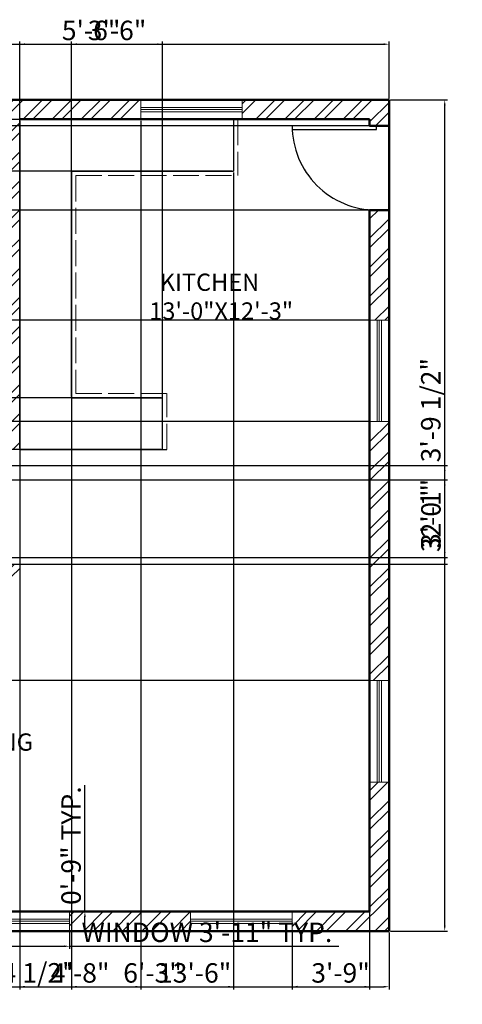
# Model space of a CAD drawing. Units: inches. Extents: x 935 to 4718, y 294 to 2318.
# Tile 2 of 2: x 1293 to 1498, y 1841 to 2297. Entities that reach past the tile are written whole.
import ezdxf

# ---------------------------------------------------------------- set-up
doc = ezdxf.new("R2010")
doc.units = ezdxf.units.IN
doc.linetypes.add('ACAD_ISO02W100', pattern=[15, 12, -3])
for name, color, linetype, lineweight in [('A-ANNO-DIMS', 2, 'Continuous', 18), ('A-AREA-IDEN', 7, 'Continuous', 25), ('A-DOOR', 4, 'Continuous', 25), ('A-FLOR-CASE', 8, 'Continuous', 25), ('A-FLOR-CASE-HIDN', 8, 'ACAD_ISO02W100', 18), ('A-GLAZ', 244, 'Continuous', 18), ('A-WALL', 7, 'Continuous', 50), ('A-WALL-PATT', 8, 'Continuous', 13)]:
    doc.layers.add(name, color=color, linetype=linetype, lineweight=lineweight)
doc.styles.get("Standard").update_dxf_attribs({"font": 'arial.ttf'})
doc.dimstyles.new('ISO-25', dxfattribs={"dimtxt": 9, "dimasz": 2.5, "dimexe": 1.25, "dimexo": 0.625, "dimtad": 1, "dimlunit": 3, "dimtxsty": 'Standard', "dimcen": 2.5, "dimadec": 0, "dimazin": 0, "dimtfac": 1, "dimtmove": 0, "dimatfit": 3, "dimfxl": 1, "dimarcsym": 0})

# ---------------------------------------------------------------- blocks, each defined once
blk = doc.blocks.new('*U5')
for p, q in [((0, 0), (0, 6)), ((40, 0), (40, 6))]:
    blk.add_line(p, q)
blk.add_lwpolyline([(0, 0), (0, -40), (1.75, -40), (1.75, 0)], close=True)
blk.add_arc((0, 0), 40, 270, 0)
blk = doc.blocks.new('WIN-47IN')
for p, q in [((0, 5.5), (47, 5.5)), ((0, 4.5), (47, 4.5)), ((0, 3.5), (47, 3.5))]:
    blk.add_line(p, q)
blk.add_lwpolyline([(0, 9), (47, 9), (47, 0), (0, 0)], close=True)
blk = doc.blocks.new('*D10')
at = {"layer": 'A-ANNO-DIMS', "color": 0, "lineweight": -2, "transparency": 16777216}
for p, q in [((1268.86, 1874.07), (1268.86, 1866.39)), ((1315.86, 1874.07), (1315.86, 1866.39)), ((1271.36, 1867.64), (1313.36, 1867.64)), ((1315.86, 1867.64), (1440.49, 1867.64))]:
    blk.add_line(p, q, dxfattribs=at)
at = {"layer": 'A-ANNO-DIMS', "color": 0, "transparency": 16777216}
for points in [[(1271.36, 1868.06), (1271.36, 1867.23), (1268.86, 1867.64)], [(1313.36, 1868.06), (1313.36, 1867.23), (1315.86, 1867.64)]]:
    blk.add_solid(points, dxfattribs=at)
at = {"layer": 'Defpoints', "color": 0, "transparency": 16777216}
for p in [(1268.86, 1874.69), (1315.86, 1874.69), (1315.86, 1867.64)]:
    blk.add_point(p, dxfattribs=at)
at = {"layer": 'A-ANNO-DIMS', "color": 0, "transparency": 16777216, "insert": (1379.42, 1872.93), "char_height": 9, "attachment_point": 5}
blk.add_mtext('WINDOW 3\'-11" TYP.', dxfattribs=at)
blk = doc.blocks.new('*D11')
at = {"layer": 'A-ANNO-DIMS', "color": 0, "lineweight": -2, "transparency": 16777216}
for p, q in [((1322.91, 1883.69), (1322.91, 1942.3)), ((1316.48, 1883.69), (1324.16, 1883.69)), ((1322.91, 1877.19), (1322.91, 1881.19)), ((1316.48, 1874.69), (1324.16, 1874.69))]:
    blk.add_line(p, q, dxfattribs=at)
at = {"layer": 'A-ANNO-DIMS', "color": 0, "transparency": 16777216}
for points in [[(1322.49, 1881.19), (1323.32, 1881.19), (1322.91, 1883.69)], [(1322.49, 1877.19), (1323.32, 1877.19), (1322.91, 1874.69)]]:
    blk.add_solid(points, dxfattribs=at)
at = {"layer": 'Defpoints', "color": 0, "transparency": 16777216}
for p in [(1315.86, 1883.69), (1322.91, 1883.69), (1315.86, 1874.69)]:
    blk.add_point(p, dxfattribs=at)
at = {"layer": 'A-ANNO-DIMS', "color": 0, "transparency": 16777216, "insert": (1317.69, 1914.25), "char_height": 9, "attachment_point": 5, "rotation": 90}
blk.add_mtext('0\'-9" TYP.', dxfattribs=at)
blk = doc.blocks.new('*D16')
at = {"layer": 'A-ANNO-DIMS', "color": 0, "lineweight": -2, "transparency": 16777216}
for p, q in [((971.73, 2260.32), (971.73, 2286.74)), ((974.23, 2285.49), (1461.23, 2285.49)), ((1463.73, 2260.32), (1463.73, 2286.74))]:
    blk.add_line(p, q, dxfattribs=at)
at = {"layer": 'A-ANNO-DIMS', "color": 0, "transparency": 16777216}
for points in [[(974.23, 2285.91), (974.23, 2285.08), (971.73, 2285.49)], [(1461.23, 2285.91), (1461.23, 2285.08), (1463.73, 2285.49)]]:
    blk.add_solid(points, dxfattribs=at)
at = {"layer": 'Defpoints', "color": 0, "transparency": 16777216}
for p in [(1463.73, 2285.49), (971.73, 2259.69), (1463.73, 2259.69)]:
    blk.add_point(p, dxfattribs=at)
at = {"layer": 'A-ANNO-DIMS', "color": 0, "transparency": 16777216, "insert": (1217.73, 2290.71), "char_height": 9, "attachment_point": 5}
blk.add_mtext('41\'-0"', dxfattribs=at)
blk = doc.blocks.new('*D17')
at = {"layer": 'A-ANNO-DIMS', "color": 0, "lineweight": -2, "transparency": 16777216}
for p, q in [((1464.35, 2259.69), (1490.78, 2259.69)), ((1489.53, 1877.19), (1489.53, 2257.19)), ((1464.35, 1874.69), (1490.78, 1874.69))]:
    blk.add_line(p, q, dxfattribs=at)
at = {"layer": 'A-ANNO-DIMS', "color": 0, "transparency": 16777216}
for points in [[(1489.11, 2257.19), (1489.94, 2257.19), (1489.53, 2259.69)], [(1489.11, 1877.19), (1489.94, 1877.19), (1489.53, 1874.69)]]:
    blk.add_solid(points, dxfattribs=at)
at = {"layer": 'Defpoints', "color": 0, "transparency": 16777216}
for p in [(1463.73, 2259.69), (1489.53, 2259.69), (1463.73, 1874.69)]:
    blk.add_point(p, dxfattribs=at)
at = {"layer": 'A-ANNO-DIMS', "color": 0, "transparency": 16777216, "insert": (1484.3, 2067.19), "char_height": 9, "attachment_point": 5, "rotation": 90}
blk.add_mtext('32\'-1"', dxfattribs=at)
blk = doc.blocks.new('*D20')
at = {"layer": 'A-ANNO-DIMS', "color": 0, "lineweight": -2, "transparency": 16777216}
for p, q in [((1292.73, 2250.07), (1292.73, 1847.64)), ((1348.75, 2250.07), (1348.75, 1847.64)), ((1295.23, 1848.89), (1346.25, 1848.89))]:
    blk.add_line(p, q, dxfattribs=at)
at = {"layer": 'A-ANNO-DIMS', "color": 0, "transparency": 16777216}
for points in [[(1295.23, 1849.31), (1295.23, 1848.48), (1292.73, 1848.89)], [(1346.25, 1849.31), (1346.25, 1848.48), (1348.75, 1848.89)]]:
    blk.add_solid(points, dxfattribs=at)
at = {"layer": 'Defpoints', "color": 0, "transparency": 16777216}
for p in [(1292.73, 2250.69), (1348.75, 2250.69), (1348.75, 1848.89)]:
    blk.add_point(p, dxfattribs=at)
at = {"layer": 'A-ANNO-DIMS', "color": 0, "transparency": 16777216, "insert": (1320.74, 1854.11), "char_height": 9, "attachment_point": 5}
blk.add_mtext('4\'-8"', dxfattribs=at)
blk = doc.blocks.new('*D24')
at = {"layer": 'A-ANNO-DIMS', "color": 0, "lineweight": -2, "transparency": 16777216}
for p, q in [((1252.46, 1874.07), (1252.46, 1847.64)), ((1268.86, 1874.07), (1268.86, 1847.64)), ((1254.96, 1848.89), (1266.36, 1848.89)), ((1268.86, 1848.89), (1316.66, 1848.89))]:
    blk.add_line(p, q, dxfattribs=at)
at = {"layer": 'A-ANNO-DIMS', "color": 0, "transparency": 16777216}
for points in [[(1254.96, 1849.31), (1254.96, 1848.48), (1252.46, 1848.89)], [(1266.36, 1849.31), (1266.36, 1848.48), (1268.86, 1848.89)]]:
    blk.add_solid(points, dxfattribs=at)
at = {"layer": 'Defpoints', "color": 0, "transparency": 16777216}
for p in [(1252.46, 1874.69), (1268.86, 1874.69), (1268.86, 1848.89)]:
    blk.add_point(p, dxfattribs=at)
at = {"layer": 'A-ANNO-DIMS', "color": 0, "transparency": 16777216, "insert": (1294.01, 1854.17), "char_height": 9, "attachment_point": 5}
blk.add_mtext('1\'-4 1/2"', dxfattribs=at)
blk = doc.blocks.new('*D25')
at = {"layer": 'A-ANNO-DIMS', "color": 0, "lineweight": -2, "transparency": 16777216}
for p, q in [((1418.86, 1874.07), (1418.86, 1847.64)), ((1463.73, 1874.07), (1463.73, 1847.64)), ((1421.36, 1848.89), (1461.23, 1848.89))]:
    blk.add_line(p, q, dxfattribs=at)
at = {"layer": 'A-ANNO-DIMS', "color": 0, "transparency": 16777216}
for points in [[(1421.36, 1849.31), (1421.36, 1848.48), (1418.86, 1848.89)], [(1461.23, 1849.31), (1461.23, 1848.48), (1463.73, 1848.89)]]:
    blk.add_solid(points, dxfattribs=at)
at = {"layer": 'Defpoints', "color": 0, "transparency": 16777216}
for p in [(1418.86, 1874.69), (1463.73, 1874.69), (1463.73, 1848.89)]:
    blk.add_point(p, dxfattribs=at)
at = {"layer": 'A-ANNO-DIMS', "color": 0, "transparency": 16777216, "insert": (1441.29, 1854.12), "char_height": 9, "attachment_point": 5}
blk.add_mtext('3\'-9"', dxfattribs=at)
blk = doc.blocks.new('*D27')
at = {"layer": 'A-ANNO-DIMS', "color": 0, "lineweight": -2, "transparency": 16777216}
for p, q in [((1489.53, 2090.41), (1489.53, 2139.04)), ((981.35, 2090.41), (1490.78, 2090.41)), ((1489.53, 2047.19), (1489.53, 2087.91)), ((981.35, 2044.69), (1490.78, 2044.69))]:
    blk.add_line(p, q, dxfattribs=at)
at = {"layer": 'A-ANNO-DIMS', "color": 0, "transparency": 16777216}
for points in [[(1489.11, 2087.91), (1489.94, 2087.91), (1489.53, 2090.41)], [(1489.11, 2047.19), (1489.94, 2047.19), (1489.53, 2044.69)]]:
    blk.add_solid(points, dxfattribs=at)
at = {"layer": 'Defpoints', "color": 0, "transparency": 16777216}
for p in [(980.73, 2090.41), (1489.53, 2090.41), (980.73, 2044.69)]:
    blk.add_point(p, dxfattribs=at)
at = {"layer": 'A-ANNO-DIMS', "color": 0, "transparency": 16777216, "insert": (1484.24, 2115.97), "char_height": 9, "attachment_point": 5, "rotation": 90}
blk.add_mtext('3\'-9 1/2"', dxfattribs=at)
blk = doc.blocks.new('*D29')
at = {"layer": 'A-ANNO-DIMS', "color": 0, "lineweight": -2, "transparency": 16777216}
for p, q in [((945.93, 2253.19), (945.93, 2255.69)), ((1454.1, 2250.69), (944.68, 2250.69)), ((945.93, 2250.69), (945.93, 2247.69)), ((1418.25, 2247.69), (944.68, 2247.69)), ((945.93, 2245.19), (945.93, 2217.52))]:
    blk.add_line(p, q, dxfattribs=at)
at = {"layer": 'A-ANNO-DIMS', "color": 0, "transparency": 16777216}
for points in [[(945.51, 2253.19), (946.34, 2253.19), (945.93, 2250.69)], [(945.51, 2245.19), (946.34, 2245.19), (945.93, 2247.69)]]:
    blk.add_solid(points, dxfattribs=at)
at = {"layer": 'Defpoints', "color": 0, "transparency": 16777216}
for p in [(1454.73, 2250.69), (945.93, 2247.69), (1418.88, 2247.69)]:
    blk.add_point(p, dxfattribs=at)
at = {"layer": 'A-ANNO-DIMS', "color": 0, "transparency": 16777216, "insert": (940.7, 2230.11), "char_height": 9, "attachment_point": 5, "rotation": 90}
blk.add_mtext('0\'-3"', dxfattribs=at)
blk = doc.blocks.new('*D30')
at = {"layer": 'A-ANNO-DIMS', "color": 0, "lineweight": -2, "transparency": 16777216}
for p, q in [((1454.1, 2110.69), (944.68, 2110.69)), ((945.93, 1993.19), (945.93, 2108.19)), ((1454.1, 1990.69), (944.68, 1990.69))]:
    blk.add_line(p, q, dxfattribs=at)
at = {"layer": 'A-ANNO-DIMS', "color": 0, "transparency": 16777216}
for points in [[(945.51, 2108.19), (946.34, 2108.19), (945.93, 2110.69)], [(945.51, 1993.19), (946.34, 1993.19), (945.93, 1990.69)]]:
    blk.add_solid(points, dxfattribs=at)
at = {"layer": 'Defpoints', "color": 0, "transparency": 16777216}
for p in [(945.93, 2110.69), (1454.73, 2110.69), (1454.73, 1990.69)]:
    blk.add_point(p, dxfattribs=at)
at = {"layer": 'A-ANNO-DIMS', "color": 0, "transparency": 16777216, "insert": (940.7, 2050.69), "char_height": 9, "attachment_point": 5, "rotation": 90}
blk.add_mtext('10\'-0"', dxfattribs=at)
blk = doc.blocks.new('*D31')
at = {"layer": 'A-ANNO-DIMS', "color": 0, "lineweight": -2, "transparency": 16777216}
for p, q in [((1454.1, 2208.69), (944.68, 2208.69)), ((945.93, 2160.19), (945.93, 2206.19)), ((1454.1, 2157.69), (944.68, 2157.69))]:
    blk.add_line(p, q, dxfattribs=at)
at = {"layer": 'A-ANNO-DIMS', "color": 0, "transparency": 16777216}
for points in [[(945.51, 2206.19), (946.34, 2206.19), (945.93, 2208.69)], [(945.51, 2160.19), (946.34, 2160.19), (945.93, 2157.69)]]:
    blk.add_solid(points, dxfattribs=at)
at = {"layer": 'Defpoints', "color": 0, "transparency": 16777216}
for p in [(945.93, 2208.69), (1454.73, 2208.69), (1454.73, 2157.69)]:
    blk.add_point(p, dxfattribs=at)
at = {"layer": 'A-ANNO-DIMS', "color": 0, "transparency": 16777216, "insert": (940.7, 2183.19), "char_height": 9, "attachment_point": 5, "rotation": 90}
blk.add_mtext('4\'-3"', dxfattribs=at)
blk = doc.blocks.new('*D32')
at = {"layer": 'A-ANNO-DIMS', "color": 0, "lineweight": -2, "transparency": 16777216}
for p, q in [((1454.1, 2247.69), (944.68, 2247.69)), ((945.93, 2211.19), (945.93, 2245.19)), ((1454.1, 2208.69), (944.68, 2208.69))]:
    blk.add_line(p, q, dxfattribs=at)
at = {"layer": 'A-ANNO-DIMS', "color": 0, "transparency": 16777216}
for points in [[(945.51, 2245.19), (946.34, 2245.19), (945.93, 2247.69)], [(945.51, 2211.19), (946.34, 2211.19), (945.93, 2208.69)]]:
    blk.add_solid(points, dxfattribs=at)
at = {"layer": 'Defpoints', "color": 0, "transparency": 16777216}
for p in [(945.93, 2247.69), (1454.73, 2247.69), (1454.73, 2208.69)]:
    blk.add_point(p, dxfattribs=at)
at = {"layer": 'A-ANNO-DIMS', "color": 0, "transparency": 16777216, "insert": (940.7, 2228.19), "char_height": 9, "attachment_point": 5, "rotation": 90}
blk.add_mtext('3\'-3"', dxfattribs=at)
blk = doc.blocks.new('*D36')
at = {"layer": 'A-ANNO-DIMS', "color": 0, "lineweight": -2, "transparency": 16777216}
for p, q in [((1454.73, 2110.07), (1454.73, 1847.64)), ((1292.73, 2097.07), (1292.73, 1847.64)), ((1295.23, 1848.89), (1452.23, 1848.89))]:
    blk.add_line(p, q, dxfattribs=at)
at = {"layer": 'A-ANNO-DIMS', "color": 0, "transparency": 16777216}
for points in [[(1295.23, 1849.31), (1295.23, 1848.48), (1292.73, 1848.89)], [(1452.23, 1849.31), (1452.23, 1848.48), (1454.73, 1848.89)]]:
    blk.add_solid(points, dxfattribs=at)
at = {"layer": 'Defpoints', "color": 0, "transparency": 16777216}
for p in [(1454.73, 2110.69), (1292.73, 2097.69), (1454.73, 1848.89)]:
    blk.add_point(p, dxfattribs=at)
at = {"layer": 'A-ANNO-DIMS', "color": 0, "transparency": 16777216, "insert": (1373.73, 1854.12), "char_height": 9, "attachment_point": 5}
blk.add_mtext('13\'-6"', dxfattribs=at)
blk = doc.blocks.new('*D37')
at = {"layer": 'A-ANNO-DIMS', "color": 0, "lineweight": -2, "transparency": 16777216}
for p, q in [((945.93, 2250.69), (945.93, 2278.52)), ((1391.1, 2250.69), (944.68, 2250.69)), ((945.93, 2229.19), (945.93, 2248.19)), ((1391.1, 2226.69), (944.68, 2226.69))]:
    blk.add_line(p, q, dxfattribs=at)
at = {"layer": 'A-ANNO-DIMS', "color": 0, "transparency": 16777216}
for points in [[(945.51, 2248.19), (946.34, 2248.19), (945.93, 2250.69)], [(945.51, 2229.19), (946.34, 2229.19), (945.93, 2226.69)]]:
    blk.add_solid(points, dxfattribs=at)
at = {"layer": 'Defpoints', "color": 0, "transparency": 16777216}
for p in [(945.93, 2250.69), (1391.73, 2250.69), (1391.73, 2226.69)]:
    blk.add_point(p, dxfattribs=at)
at = {"layer": 'A-ANNO-DIMS', "color": 0, "transparency": 16777216, "insert": (940.7, 2265.86), "char_height": 9, "attachment_point": 5, "rotation": 90}
blk.add_mtext('2\'-0"', dxfattribs=at)
blk = doc.blocks.new('*D38')
at = {"layer": 'A-ANNO-DIMS', "color": 0, "lineweight": -2, "transparency": 16777216}
for p, q in [((1316.73, 2226.07), (1316.73, 1847.64)), ((1391.73, 2226.07), (1391.73, 1847.64)), ((1319.23, 1848.89), (1389.23, 1848.89))]:
    blk.add_line(p, q, dxfattribs=at)
at = {"layer": 'A-ANNO-DIMS', "color": 0, "transparency": 16777216}
for points in [[(1319.23, 1849.31), (1319.23, 1848.48), (1316.73, 1848.89)], [(1389.23, 1849.31), (1389.23, 1848.48), (1391.73, 1848.89)]]:
    blk.add_solid(points, dxfattribs=at)
at = {"layer": 'Defpoints', "color": 0, "transparency": 16777216}
for p in [(1316.73, 2226.69), (1391.73, 2226.69), (1391.73, 1848.89)]:
    blk.add_point(p, dxfattribs=at)
at = {"layer": 'A-ANNO-DIMS', "color": 0, "transparency": 16777216, "insert": (1354.23, 1854.12), "char_height": 9, "attachment_point": 5}
blk.add_mtext('6\'-3"', dxfattribs=at)
blk = doc.blocks.new('*D39')
at = {"layer": 'A-ANNO-DIMS', "color": 0, "lineweight": -2, "transparency": 16777216}
for p, q in [((1292.73, 2098.32), (1292.73, 2286.74)), ((1295.23, 2285.49), (1356.38, 2285.49)), ((1358.88, 2098.32), (1358.88, 2286.74))]:
    blk.add_line(p, q, dxfattribs=at)
at = {"layer": 'A-ANNO-DIMS', "color": 0, "transparency": 16777216}
for points in [[(1295.23, 2285.91), (1295.23, 2285.08), (1292.73, 2285.49)], [(1356.38, 2285.91), (1356.38, 2285.08), (1358.88, 2285.49)]]:
    blk.add_solid(points, dxfattribs=at)
at = {"layer": 'Defpoints', "color": 0, "transparency": 16777216}
for p in [(1358.88, 2285.49), (1292.73, 2097.69), (1358.88, 2097.69)]:
    blk.add_point(p, dxfattribs=at)
at = {"layer": 'A-ANNO-DIMS', "color": 0, "transparency": 16777216, "insert": (1325.8, 2290.71), "char_height": 9, "attachment_point": 5}
blk.add_mtext('5\'-6"', dxfattribs=at)
blk = doc.blocks.new('*D40')
at = {"layer": 'A-ANNO-DIMS', "color": 0, "lineweight": -2, "transparency": 16777216}
for p, q in [((1316.73, 2122.32), (1316.73, 2286.74)), ((1319.23, 2285.49), (1356.38, 2285.49)), ((1358.88, 2122.32), (1358.88, 2286.74))]:
    blk.add_line(p, q, dxfattribs=at)
at = {"layer": 'A-ANNO-DIMS', "color": 0, "transparency": 16777216}
for points in [[(1319.23, 2285.91), (1319.23, 2285.08), (1316.73, 2285.49)], [(1356.38, 2285.91), (1356.38, 2285.08), (1358.88, 2285.49)]]:
    blk.add_solid(points, dxfattribs=at)
at = {"layer": 'Defpoints', "color": 0, "transparency": 16777216}
for p in [(1358.88, 2285.49), (1316.73, 2121.69), (1358.88, 2121.69)]:
    blk.add_point(p, dxfattribs=at)
at = {"layer": 'A-ANNO-DIMS', "color": 0, "transparency": 16777216, "insert": (1337.8, 2290.72), "char_height": 9, "attachment_point": 5}
blk.add_mtext('3\'-6"', dxfattribs=at)
blk = doc.blocks.new('*D41')
at = {"layer": 'A-ANNO-DIMS', "color": 0, "lineweight": -2, "transparency": 16777216}
for p, q in [((1358.25, 2121.69), (944.68, 2121.69)), ((945.93, 2119.19), (945.93, 2100.19)), ((1358.25, 2097.69), (944.68, 2097.69)), ((945.93, 2097.69), (945.93, 2069.87))]:
    blk.add_line(p, q, dxfattribs=at)
at = {"layer": 'A-ANNO-DIMS', "color": 0, "transparency": 16777216}
for points in [[(945.51, 2119.19), (946.34, 2119.19), (945.93, 2121.69)], [(945.51, 2100.19), (946.34, 2100.19), (945.93, 2097.69)]]:
    blk.add_solid(points, dxfattribs=at)
at = {"layer": 'Defpoints', "color": 0, "transparency": 16777216}
for p in [(1358.88, 2121.69), (945.93, 2097.69), (1358.88, 2097.69)]:
    blk.add_point(p, dxfattribs=at)
at = {"layer": 'A-ANNO-DIMS', "color": 0, "transparency": 16777216, "insert": (940.7, 2082.53), "char_height": 9, "attachment_point": 5, "rotation": 90}
blk.add_mtext('2\'-0"', dxfattribs=at)
blk = doc.blocks.new('*D42')
at = {"layer": 'A-ANNO-DIMS', "color": 0, "lineweight": -2, "transparency": 16777216}
for p, q in [((1095.35, 2083.69), (1490.78, 2083.69)), ((1489.53, 2050.19), (1489.53, 2081.19)), ((1095.35, 2047.69), (1490.78, 2047.69))]:
    blk.add_line(p, q, dxfattribs=at)
at = {"layer": 'A-ANNO-DIMS', "color": 0, "transparency": 16777216}
for points in [[(1489.11, 2081.19), (1489.94, 2081.19), (1489.53, 2083.69)], [(1489.11, 2050.19), (1489.94, 2050.19), (1489.53, 2047.69)]]:
    blk.add_solid(points, dxfattribs=at)
at = {"layer": 'Defpoints', "color": 0, "transparency": 16777216}
for p in [(1094.73, 2083.69), (1489.53, 2083.69), (1094.73, 2047.69)]:
    blk.add_point(p, dxfattribs=at)
at = {"layer": 'A-ANNO-DIMS', "color": 0, "transparency": 16777216, "insert": (1484.3, 2065.69), "char_height": 9, "attachment_point": 5, "rotation": 90}
blk.add_mtext('3\'-0"', dxfattribs=at)

msp = doc.modelspace()

# ---------------------------------------------------------------- hatches: boundary and pattern name
at = {"layer": 'A-WALL-PATT'}
h = msp.add_hatch(dxfattribs=at)
h.set_pattern_fill('ANSI32', color=256)
h.paths.add_polyline_path([(1292.725, 2044.693), (1131.725, 2044.693), (1131.725, 2038.693), (1134.725, 2038.693), (1134.725, 1883.693), (1083.516, 1883.693), (1083.516, 1874.693), (1213.462, 1874.693), (1213.462, 1883.693), (1140.725, 1883.693), (1140.725, 2038.693), (1292.725, 2038.693)])
h.paths.add_polyline_path([(1463.725, 1943.693), (1454.725, 1943.693), (1454.725, 1883.693), (1418.857, 1883.693), (1418.857, 1874.693), (1463.725, 1874.693)])
h.paths.add_polyline_path([(1463.725, 2110.693), (1454.725, 2110.693), (1454.725, 1990.693), (1463.725, 1990.693)])
h.paths.add_polyline_path([(1371.857, 1883.693), (1315.857, 1883.693), (1315.857, 1874.693), (1371.857, 1874.693)])
h.paths.add_polyline_path([(1036.516, 1883.693), (980.725, 1883.693), (980.725, 1937.693), (971.725, 1937.693), (971.725, 1874.693), (1036.516, 1874.693)])
h.paths.add_polyline_path([(980.725, 2038.693), (1094.725, 2038.693), (1095.725, 2038.693), (1095.725, 2044.093), (1095.725, 2044.693), (1094.725, 2044.693), (1094.725, 2047.693), (1088.725, 2047.693), (1088.725, 2044.693), (980.725, 2044.693), (980.725, 2090.405), (971.725, 2090.405), (971.725, 1984.693), (980.725, 1984.693)])
h.paths.add_polyline_path([(1292.725, 2250.693), (1348.753, 2250.693), (1348.753, 2259.693), (1238.771, 2259.693), (1238.771, 2250.693), (1286.725, 2250.693), (1286.725, 2103.693), (1133.725, 2103.693), (1133.725, 2097.693), (1292.725, 2097.693)])
h.paths.add_polyline_path([(1463.725, 2208.693), (1457.875, 2208.693), (1454.725, 2208.693), (1454.725, 2157.693), (1463.725, 2157.693)])
h.paths.add_polyline_path([(1463.725, 2259.693), (1395.753, 2259.693), (1395.753, 2250.693), (1454.725, 2250.693), (1454.725, 2247.693), (1457.875, 2247.693), (1463.725, 2247.693)])
h.paths.add_polyline_path([(1203.771, 2259.693), (1140.771, 2259.693), (1140.771, 2250.693), (1203.771, 2250.693)], flags=17)
h.paths.add_polyline_path([(1105.771, 2259.693), (971.725, 2259.693), (971.725, 2194.405), (980.725, 2194.405), (980.725, 2250.693), (1088.725, 2250.693), (1088.725, 2247.693), (1091.725, 2247.693), (1094.725, 2247.693), (1094.725, 2250.693), (1105.771, 2250.693)])
h.paths.add_polyline_path([(1094.725, 2211.693), (1088.725, 2211.693), (1088.725, 2149.693), (980.725, 2149.693), (980.725, 2170.405), (971.725, 2170.405), (971.725, 2114.405), (980.725, 2114.405), (980.725, 2143.693), (1088.725, 2143.693), (1088.725, 2083.693), (1091.725, 2083.693), (1094.725, 2083.693), (1094.725, 2097.693), (1097.725, 2097.693), (1097.725, 2103.693), (1094.725, 2103.693)])

# ---------------------------------------------------------------- linework, layer by layer
at = {"layer": 'A-FLOR-CASE'}
for p, q in [((1391.725, 2250.693), (1391.725, 2226.693)), ((1316.725, 2226.693), (1316.725, 2121.693)), ((1316.725, 2226.693), (1391.725, 2226.693)), ((1316.725, 2121.693), (1358.876, 2121.693)), ((1358.876, 2097.693), (1358.876, 2121.693)), ((1292.725, 2097.693), (1360.876, 2097.693))]:
    msp.add_line(p, q, dxfattribs=at)
at = {"layer": 'A-FLOR-CASE-HIDN'}
for p, q in [((1393.725, 2250.693), (1393.725, 2224.693)), ((1318.725, 2224.693), (1393.725, 2224.693)), ((1318.725, 2224.693), (1318.725, 2123.693)), ((1318.725, 2123.693), (1360.876, 2123.693)), ((1360.876, 2097.693), (1360.876, 2123.693))]:
    msp.add_line(p, q, dxfattribs=at)
at = {"layer": 'A-WALL'}
for p, q in [((971.725, 2259.693), (1463.725, 2259.693)), ((1463.725, 2259.693), (1463.725, 1874.693)), ((1292.725, 2250.693), (1454.725, 2250.693)), ((1454.725, 2250.693), (1454.725, 2247.693)), ((1454.725, 2247.693), (1463.725, 2247.693)), ((1454.725, 2208.693), (1463.725, 2208.693)), ((1454.725, 2208.693), (1454.725, 1883.693)), ((1252.462, 1883.693), (1454.725, 1883.693)), ((971.725, 1874.693), (1463.725, 1874.693))]:
    msp.add_line(p, q, dxfattribs=at)

# ---------------------------------------------------------------- block references
at = {"layer": 'A-DOOR', "xscale": 0.975, "yscale": 0.975, "zscale": 0.975, "rotation": 270}
msp.add_blockref('*U5', (1457.875, 2247.693), dxfattribs=at)
at = {"layer": 'A-GLAZ'}
for p in [(1348.753, 2250.693), (1268.857, 1874.693), (1371.857, 1874.693)]:
    msp.add_blockref('WIN-47IN', p, dxfattribs=at)
for p, rotation in [((1463.725, 2110.693), 90.00000000000146), ((1463.725, 1943.693), 90.00000000000156)]:
    msp.add_blockref('WIN-47IN', p, dxfattribs=dict(at, rotation=rotation))

# ---------------------------------------------------------------- texts
at = {"layer": 'A-AREA-IDEN', "char_height": 8, "attachment_point": 1}
for s, width, insert in [('  KITCHEN\\P13\'-0"X12\'-3"', 63.75514, (1352.713, 2179.235)), ('LIVING AND DINING', 119.49406, (1200.713, 1966.235))]:
    msp.add_mtext_dynamic_manual_height_columns(s, width=width, gutter_width=12.5, heights=[0], dxfattribs=dict(at, insert=insert))

# ---------------------------------------------------------------- dimensions: what is measured, and where the dimension line sits
at = {"layer": 'A-ANNO-DIMS'}
for base, p1, p2, picture, middle in [((1463.725, 2285.493), (971.725, 2259.693), (1463.725, 2259.693), '*D16', (1217.725, 2290.713)), ((1358.876, 2285.493), (1292.725, 2097.693), (1358.876, 2097.693), '*D39', (1325.801, 2290.713)), ((1358.876, 2285.493), (1316.725, 2121.693), (1358.876, 2121.693), '*D40', (1337.801, 2290.716)), ((1348.753, 1848.893), (1292.725, 2250.693), (1348.753, 2250.693), '*D20', (1320.739, 1854.113)), ((1391.725, 1848.893), (1316.725, 2226.693), (1391.725, 2226.693), '*D38', (1354.225, 1854.116)), ((1454.725, 1848.893), (1292.725, 2097.693), (1454.725, 2110.693), '*D36', (1373.725, 1854.116)), ((1268.857, 1848.893), (1252.462, 1874.693), (1268.857, 1874.693), '*D24', (1294.006, 1854.171)), ((1463.725, 1848.893), (1418.857, 1874.693), (1463.725, 1874.693), '*D25', (1441.291, 1854.116))]:
    dim = msp.add_linear_dim(base=base, p1=p1, p2=p2, dimstyle='ISO-25', override={"dimdec": 1, "dimlfac": 1, "dimrnd": 0, "dimzin": 1, "dimdsep": 46, "dimlunit": 4, "dimfrac": 2}, dxfattribs=at)
    dim.commit()
    dim.dimension.update_dxf_attribs({"geometry": picture, "text_midpoint": middle})
for base, p1, p2, picture, middle in [((945.925, 2250.693), (1391.725, 2226.693), (1391.725, 2250.693), '*D37', (940.705, 2265.857)), ((1489.525, 2259.693), (1463.725, 1874.693), (1463.725, 2259.693), '*D17', (1484.302, 2067.193)), ((945.925, 2247.693), (1454.725, 2250.693), (1418.875, 2247.693), '*D29', (940.702, 2230.106)), ((945.925, 2247.693), (1454.725, 2208.693), (1454.725, 2247.693), '*D32', (940.702, 2228.193)), ((945.925, 2208.693), (1454.725, 2157.693), (1454.725, 2208.693), '*D31', (940.702, 2183.193)), ((1489.525, 2090.405), (980.725, 2044.693), (980.725, 2090.405), '*D27', (1484.244, 2115.975)), ((945.925, 2097.693), (1358.876, 2121.693), (1358.876, 2097.693), '*D41', (940.705, 2082.529)), ((945.925, 2110.693), (1454.725, 1990.693), (1454.725, 2110.693), '*D30', (940.705, 2050.693)), ((1489.525, 2083.693), (1094.725, 2047.693), (1094.725, 2083.693), '*D42', (1484.302, 2065.693))]:
    dim = msp.add_linear_dim(base=base, p1=p1, p2=p2, angle=90, dimstyle='ISO-25', override={"dimdec": 1, "dimlfac": 1, "dimrnd": 0, "dimzin": 1, "dimdsep": 46, "dimlunit": 4, "dimfrac": 2}, dxfattribs=at)
    dim.commit()
    dim.dimension.update_dxf_attribs({"geometry": picture, "text_midpoint": middle})
dim = msp.add_linear_dim(base=(1322.907, 1883.693), p1=(1315.857, 1874.693), p2=(1315.857, 1883.693), angle=90, text='<> TYP.', dimstyle='ISO-25', override={"dimdec": 1, "dimlfac": 1, "dimrnd": 0, "dimzin": 1, "dimdsep": 46, "dimlunit": 4, "dimfrac": 2}, dxfattribs=at)
dim.commit()
dim.dimension.update_dxf_attribs({"geometry": '*D11', "text_midpoint": (1317.687, 1914.248)})
dim = msp.add_linear_dim(base=(1315.857, 1867.643), p1=(1268.857, 1874.693), p2=(1315.857, 1874.693), text='WINDOW <> TYP.', dimstyle='ISO-25', override={"dimdec": 1, "dimlfac": 1, "dimrnd": 0, "dimzin": 1, "dimdsep": 46, "dimlunit": 4, "dimfrac": 2}, dxfattribs=at)
dim.commit()
dim.dimension.update_dxf_attribs({"geometry": '*D10', "text_midpoint": (1379.422, 1872.928)})

doc.saveas('drawing.dxf')
